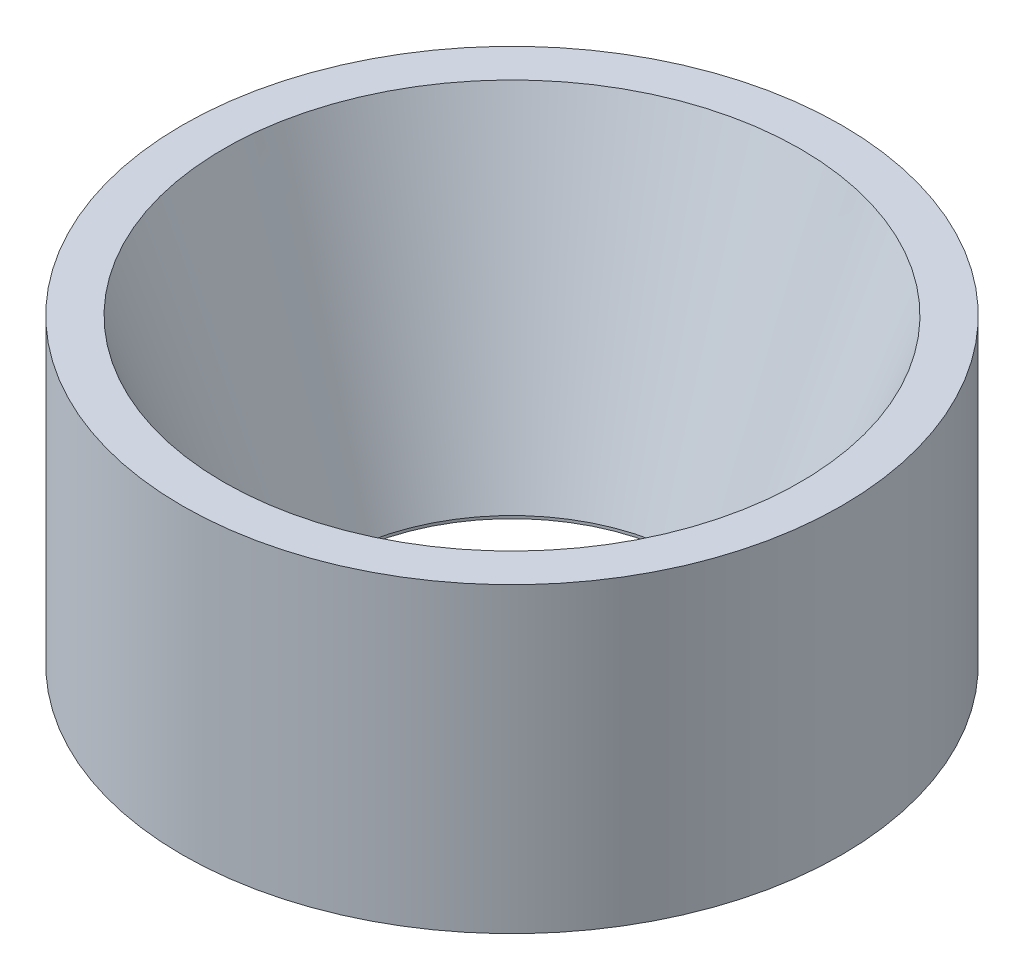
from build123d import *

# Parameters (mm, degrees)
RING_OUTLINE_SKETCH_48_R  = 24
RING_BODY_48X22_DEPTH     = 22
TAPER_TOP_PROFILE_40_R    = 21
TAPER_BOTTOM_PROFILE_20_R = 13
THROUGH_BORE_20_REACH     = 42.339
THROUGH_BORE_SKETCH_20_R  = 13


with BuildPart() as part:
    # Ring Outline Sketch Ø48 → Ring Body Ø48x22 (new body)
    with BuildSketch(Plane(origin=(0, 0, 0), x_dir=(1, 0, 0), z_dir=(0, 1, 0))):
        with Locations(Location((0, 0, 0), (0, 0, 270))):
            Circle(RING_OUTLINE_SKETCH_48_R)
    extrude(amount=RING_BODY_48X22_DEPTH)

    # Taper Top Profile Ø40 → Conical Bore Ø40-Ø20 section 0
    with BuildSketch(Plane(origin=(0, 22, 0), x_dir=(1, 0, 0), z_dir=(0, 1, 0))):
        Circle(TAPER_TOP_PROFILE_40_R)
    # Taper Bottom Profile Ø20 → Conical Bore Ø40-Ø20 section 1
    with BuildSketch(Plane(origin=(0, 0.2, 0), x_dir=(1, 0, 0), z_dir=(0, 1, 0))):
        Circle(TAPER_BOTTOM_PROFILE_20_R)
    loft(mode=Mode.SUBTRACT)

    # Through Bore Sketch Ø20 → Through Bore Ø20 (cut, up to next)
    with BuildSketch(Plane(origin=(0, 0.2, 0), x_dir=(1, 0, 0), z_dir=(0, 1, 0)), mode=Mode.PRIVATE) as through_bore_20_sk1:
        with Locations(Location((0, 0, 0), (0, 0, 270))):
            Circle(THROUGH_BORE_SKETCH_20_R)
    through_bore_20_tool1 = extrude(through_bore_20_sk1.sketch, amount=-THROUGH_BORE_20_REACH, mode=Mode.PRIVATE) & part.part
    add(through_bore_20_tool1.solids().sort_by_distance((0, 0.2, 0))[0], mode=Mode.SUBTRACT)


solid = part.part
